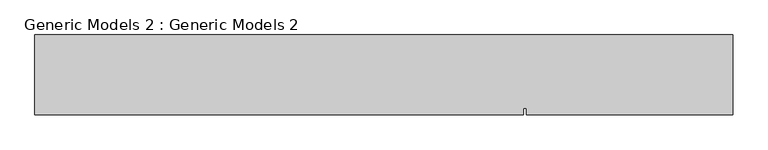
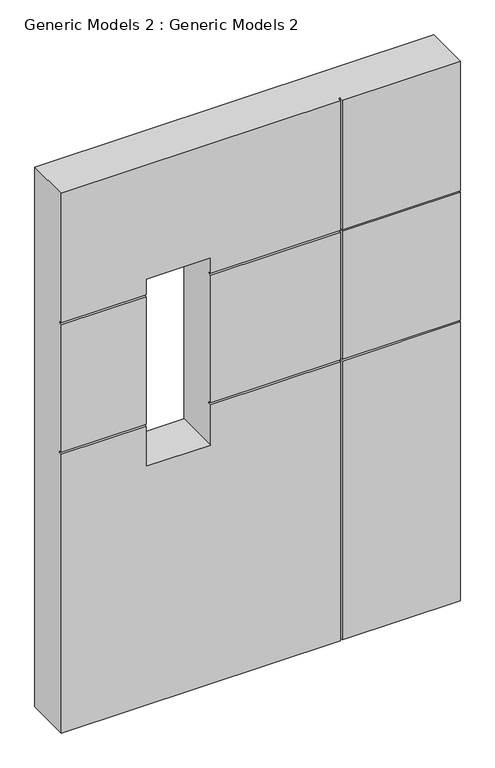
"""IFC4 building model written with IfcOpenShell, lengths in millimetres: proxy geometry, Generic Models 2 : Generic Models 2."""

from ifc_helpers import new_model, si_unit, origin, place, context, project, spatial, faceted_brep, source, transform, mapped, element, save


def generic_models_2_generic_models_2_020848e7(model_context):
    return source(origin(), model_context, "Body", "Brep", [
        faceted_brep([(-8334.9678816, 1031.7030358, 6553.2), (-10200.7615604, 1031.7030358, 6553.2), (-10200.7615604, 1031.7030358, 5638.8), (-9634.2500083, 1031.7030358, 5638.8), (-9634.2500083, 1031.7030358, 5747.6407527), (-9202.4500083, 1031.7030358, 5747.6407527), (-9202.4500083, 1031.7030358, 5638.8), (-8334.9678816, 1031.7030358, 5638.8), (-7534.8678816, 1031.7030358, 6553.2), (-8322.2678816, 1031.7030358, 6553.2), (-8322.2678816, 1031.7030358, 5638.8), (-7534.8678816, 1031.7030358, 5638.8), (-10200.7615604, 1031.7030358, 2743.2), (-8334.9678816, 1031.7030358, 2743.2), (-8334.9678816, 1031.7030358, 4711.7), (-9202.4500083, 1031.7030358, 4711.7), (-9202.4500083, 1031.7030358, 4426.8407527), (-9634.2500083, 1031.7030358, 4426.8407527), (-9634.2500083, 1031.7030358, 4711.7), (-10200.7615604, 1031.7030358, 4711.7), (-8322.2678816, 1031.7030358, 2743.2), (-7534.8678816, 1031.7030358, 2743.2), (-7534.8678816, 1031.7030358, 4711.7), (-8322.2678816, 1031.7030358, 4711.7), (-7534.8678816, 1031.7030358, 4724.4), (-7534.8678816, 1031.7030358, 5626.1), (-8322.2678816, 1031.7030358, 5626.1), (-8322.2678816, 1031.7030358, 4724.4), (-10200.7615604, 1031.7030358, 5626.1), (-10200.7615604, 1031.7030358, 4724.4), (-9634.2500083, 1031.7030358, 4724.4), (-9634.2500083, 1031.7030358, 5626.1), (-8334.9678816, 1031.7030358, 4724.4), (-8334.9678816, 1031.7030358, 5626.1), (-9202.4500083, 1031.7030358, 5626.1), (-9202.4500083, 1031.7030358, 4724.4), (-7534.8678816, 1336.5030358, 2743.2), (-10200.7615604, 1336.5030358, 2743.2), (-10200.7615604, 1336.5030358, 6553.2), (-7534.8678816, 1336.5030358, 6553.2), (-9202.4500083, 1336.5030358, 4426.8407527), (-9202.4500083, 1336.5030358, 5747.6407527), (-9634.2500083, 1336.5030358, 5747.6407527), (-9634.2500083, 1336.5030358, 4426.8407527), (-7534.8678816, 1057.1030358, 5638.8), (-7534.8678816, 1057.1030358, 5626.1), (-7534.8678816, 1057.1030358, 4724.4), (-7534.8678816, 1057.1030358, 4711.7), (-8334.9678816, 1057.1030358, 6553.2), (-8322.2678816, 1057.1030358, 6553.2), (-10200.7615604, 1057.1030358, 4711.7), (-10200.7615604, 1057.1030358, 4724.4), (-10200.7615604, 1057.1030358, 5626.1), (-10200.7615604, 1057.1030358, 5638.8), (-8322.2678816, 1057.1030358, 2743.2), (-8334.9678816, 1057.1030358, 2743.2), (-8334.9678816, 1057.1030358, 5638.8), (-9202.4500083, 1057.1030358, 5638.8), (-9202.4500083, 1057.1030358, 5626.1), (-8334.9678816, 1057.1030358, 5626.1), (-8334.9678816, 1057.1030358, 4724.4), (-9202.4500083, 1057.1030358, 4724.4), (-9202.4500083, 1057.1030358, 4711.7), (-8334.9678816, 1057.1030358, 4711.7), (-8322.2678816, 1057.1030358, 4711.7), (-8322.2678816, 1057.1030358, 4724.4), (-8322.2678816, 1057.1030358, 5626.1), (-8322.2678816, 1057.1030358, 5638.8), (-9634.2500083, 1057.1030358, 4711.7), (-9634.2500083, 1057.1030358, 4724.4), (-9634.2500083, 1057.1030358, 5626.1), (-9634.2500083, 1057.1030358, 5638.8)], [[[0, 1, 2, 3, 4, 5, 6, 7]], [[8, 9, 10, 11]], [[12, 13, 14, 15, 16, 17, 18, 19]], [[20, 21, 22, 23]], [[24, 25, 26, 27]], [[28, 29, 30, 31]], [[32, 33, 34, 35]], [[36, 37, 38, 39], [40, 41, 42, 43]], [[36, 39, 8, 11, 44, 45, 25, 24, 46, 47, 22, 21]], [[39, 38, 1, 0, 48, 49, 9, 8]], [[38, 37, 12, 19, 50, 51, 29, 28, 52, 53, 2, 1]], [[37, 36, 21, 20, 54, 55, 13, 12]], [[49, 48, 56, 57, 58, 59, 60, 61, 62, 63, 55, 54, 64, 47, 46, 65, 66, 45, 44, 67]], [[51, 50, 68, 69]], [[53, 52, 70, 71]], [[33, 32, 60, 59]], [[48, 0, 7, 56]], [[13, 55, 63, 14]], [[27, 26, 66, 65]], [[9, 49, 67, 10]], [[54, 20, 23, 64]], [[52, 28, 31, 70]], [[45, 66, 26, 25]], [[33, 59, 58, 34]], [[2, 53, 71, 3]], [[67, 44, 11, 10]], [[56, 7, 6, 57]], [[50, 19, 18, 68]], [[47, 64, 23, 22]], [[14, 63, 62, 15]], [[29, 51, 69, 30]], [[65, 46, 24, 27]], [[60, 32, 35, 61]], [[40, 16, 15, 62, 61, 35, 34, 58, 57, 6, 5, 41]], [[16, 40, 43, 17]], [[17, 43, 42, 4, 3, 71, 70, 31, 30, 69, 68, 18]], [[41, 5, 4, 42]]]),
    ])


if __name__ == "__main__":
    model = new_model("IFC4")
    model_context = context("Model", 3, world=origin())
    ifc_project = project(units=[si_unit("LENGTHUNIT", "METRE", prefix="MILLI")], contexts=[model_context])
    site = spatial("IfcSite", under=ifc_project)
    building = spatial("IfcBuilding", under=site)
    placement = place(None, origin())
    generic_models_2_generic_models_2_shape = generic_models_2_generic_models_2_020848e7(model_context)
    element("IfcBuildingElementProxy", 1, Name="Generic Models 2 : Generic Models 2", ObjectType="Generic Models 2 : Generic Models 2", at=placement, inside=building, context=model_context, shape_type="MappedRepresentation", body=[
        mapped(generic_models_2_generic_models_2_shape, transform((0.0, 0.0, 0.0), x_axis=(1.0, 0.0, 0.0), y_axis=(0.0, 1.0, 0.0), z_axis=(0.0, 0.0, 1.0))),
    ])
    save(model, "model.ifc")

# Revit data of these elements
# Element 1 (IfcBuildingElementProxy, "Generic Models 2 : Generic Models 2")
#   Materials on its faces: "wall paint"
# Materials
#   "wall paint": class "Generic", colour RGB 120 120 120, transparency 0, Cost = 0
